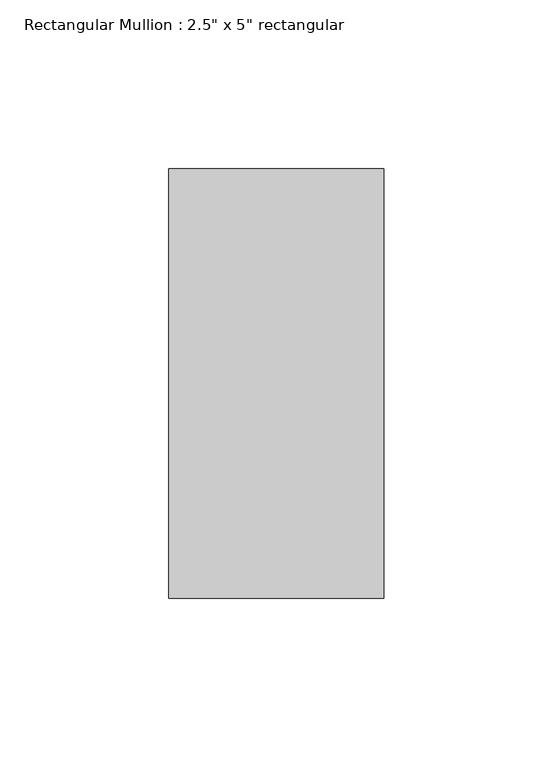
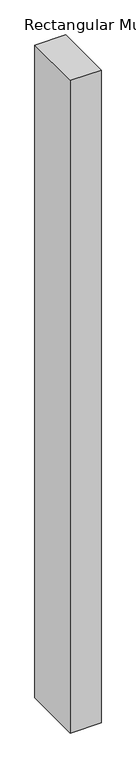
"""IFC4 building model written with IfcOpenShell, lengths in millimetres: member geometry."""

from ifc_helpers import new_model, si_unit, frame, origin, place, context, project, spatial, polyline, outline, extrude, source, transform, mapped, element, save


def member_6df10a9f(model_context):
    return source(origin(), model_context, "Body", "SweptSolid", [
        extrude(outline(polyline([(31.75, 63.5), (31.75, -63.5), (-31.75, -63.5), (-31.75, 63.5), (31.75, 63.5)])), frame((0.0, 0.0, -1428.75), z_axis=(0.0, 0.0, 1.0), x_axis=(1.0, 0.0, 0.0)), (0.0, 0.0, 1.0), 1428.75),
    ])


if __name__ == "__main__":
    model = new_model("IFC4")
    model_context = context("Model", 3, world=origin())
    ifc_project = project(units=[si_unit("LENGTHUNIT", "METRE", prefix="MILLI")], contexts=[model_context])
    site = spatial("IfcSite", under=ifc_project)
    building = spatial("IfcBuilding", under=site)
    placement = place(None, origin())
    member_shape = member_6df10a9f(model_context)
    element("IfcMember", 1, ObjectType="Rectangular Mullion : 2.5\" x 5\" rectangular", at=placement, inside=building, context=model_context, shape_type="MappedRepresentation", body=[
        mapped(member_shape, transform((0.0, 0.0, 0.0), x_axis=(1.0, 0.0, 0.0), y_axis=(0.0, 1.0, 0.0), z_axis=(0.0, 0.0, 1.0))),
    ])
    save(model, "model.ifc")

# Revit data of these elements
# Type "Rectangular Mullion : 2.5\" x 5\" rectangular"
#   built-in parameter 1007304 = 0.416667 (stored number, unit not read)
#   built-in parameter 1007301 = 0.104167 (stored number, unit not read)
#   built-in parameter 1007300 = 0.104167 (stored number, unit not read)
# Element 1 (IfcMember, "Rectangular Mullion : 2.5\" x 5\" rectangular")
#   Materials on its faces: "Rectangle 1 sq"
# Materials
#   "Rectangle 1 sq": class "Generic", colour RGB 120 120 120, transparency 0, Cost = 0
